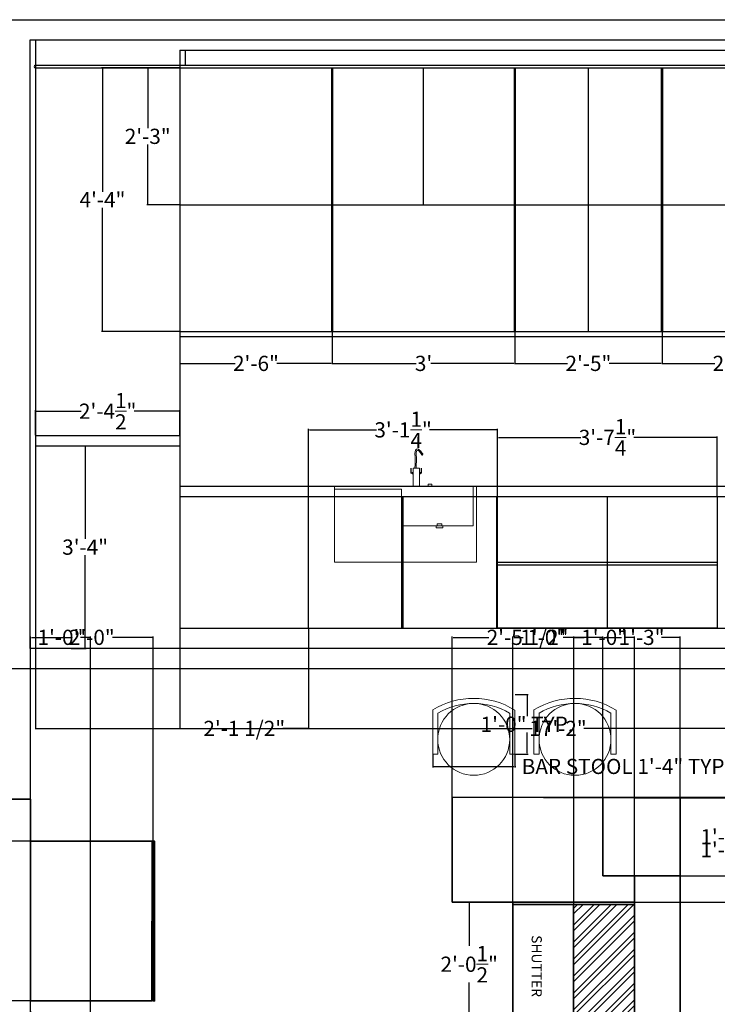
# Model space of a CAD drawing. Units: inches. Extents: x 1686244 to 1686928, y 1936095 to 1936489.
# Tile 8 of 11: x 1686478 to 1686616, y 1936281 to 1936475. Entities that reach past the tile are written whole.
import ezdxf

# ---------------------------------------------------------------- set-up
doc = ezdxf.new("R2010")
doc.units = ezdxf.units.IN
doc.header["$MEASUREMENT"] = 0
for name, color, linetype, lineweight in [('A-ANNO-DIMS', 240, 'Continuous', 18), ('A-ANNO-TEXT', 7, 'Continuous', 18), ('A-CASE', 7, 'Continuous', 35), ('A-ELEV', 7, 'Continuous', 25), ('A-FLOR-PATT', 252, 'Continuous', 13), ('A-FURN', 40, 'Continuous', 18)]:
    doc.layers.add(name, color=color, linetype=linetype, lineweight=lineweight)
doc.styles.get("Standard").update_dxf_attribs({"font": 'arial.ttf'})
doc.dimstyles.get("Standard").update_dxf_attribs({"dimtxt": 3, "dimasz": 0.18, "dimexe": 0.18, "dimexo": 0.0625, "dimgap": 0.09, "dimtad": 0, "dimtih": 1, "dimtoh": 1, "dimzin": 0, "dimdsep": 46, "dimlunit": 4, "dimtxsty": 'Standard', "dimcen": 0.09, "dimadec": 0, "dimazin": 0, "dimtfac": 1, "dimtofl": 0, "dimtmove": 0, "dimatfit": 3, "dimfxl": 1, "dimtolj": 1, "dimtzin": 0, "dimarcsym": 0})

# ---------------------------------------------------------------- blocks, each defined once
blk = doc.blocks.new('*D10')
at = {"layer": 'A-ANNO-DIMS', "color": 0, "lineweight": -2, "transparency": 16777216}
for p, q in [((1686488.94, 1936390.86), (1686491.24, 1936390.86)), ((1686491.06, 1936390.68), (1686491.06, 1936372.49)), ((1686491.06, 1936351.04), (1686491.06, 1936369.24)), ((1686488.32, 1936350.86), (1686491.24, 1936350.86))]:
    blk.add_line(p, q, dxfattribs=at)
at = {"layer": 'A-ANNO-DIMS', "color": 0, "transparency": 16777216}
for points in [[(1686491.03, 1936390.68), (1686491.09, 1936390.68), (1686491.06, 1936390.86)], [(1686491.03, 1936351.04), (1686491.09, 1936351.04), (1686491.06, 1936350.86)]]:
    blk.add_solid(points, dxfattribs=at)
at = {"layer": 'Defpoints', "color": 0, "transparency": 16777216}
for p in [(1686488.88, 1936390.86), (1686491.06, 1936390.86), (1686488.26, 1936350.86)]:
    blk.add_point(p, dxfattribs=at)
at = {"layer": 'A-ANNO-DIMS', "color": 0, "transparency": 16777216, "insert": (1686491.06, 1936370.86), "char_height": 3, "attachment_point": 5}
blk.add_mtext('\\A1;3\'-4"', dxfattribs=at)
blk = doc.blocks.new('*D11')
at = {"layer": 'A-ANNO-DIMS', "color": 0, "lineweight": -2, "transparency": 16777216}
for p, q in [((1686509.7, 1936465.36), (1686494.3, 1936465.36)), ((1686494.48, 1936465.18), (1686494.48, 1936440.95)), ((1686494.48, 1936413.54), (1686494.48, 1936437.77)), ((1686509.7, 1936413.36), (1686494.3, 1936413.36))]:
    blk.add_line(p, q, dxfattribs=at)
at = {"layer": 'A-ANNO-DIMS', "color": 0, "transparency": 16777216}
for points in [[(1686494.45, 1936465.18), (1686494.51, 1936465.18), (1686494.48, 1936465.36)], [(1686494.45, 1936413.54), (1686494.51, 1936413.54), (1686494.48, 1936413.36)]]:
    blk.add_solid(points, dxfattribs=at)
at = {"layer": 'Defpoints', "color": 0, "transparency": 16777216}
for p in [(1686509.76, 1936465.36), (1686494.48, 1936413.36), (1686509.76, 1936413.36)]:
    blk.add_point(p, dxfattribs=at)
at = {"layer": 'A-ANNO-DIMS', "color": 0, "transparency": 16777216, "insert": (1686494.48, 1936439.36), "char_height": 3, "attachment_point": 5}
blk.add_mtext('\\A1;4\'-4"', dxfattribs=at)
blk = doc.blocks.new('*D12')
at = {"layer": 'A-ANNO-DIMS', "color": 0, "lineweight": -2, "transparency": 16777216}
for p, q in [((1686509.63, 1936465.36), (1686503.22, 1936465.36)), ((1686503.4, 1936465.18), (1686503.4, 1936453.49)), ((1686503.4, 1936438.54), (1686503.4, 1936450.24)), ((1686509.7, 1936438.36), (1686503.22, 1936438.36))]:
    blk.add_line(p, q, dxfattribs=at)
at = {"layer": 'A-ANNO-DIMS', "color": 0, "transparency": 16777216}
for points in [[(1686503.37, 1936465.18), (1686503.43, 1936465.18), (1686503.4, 1936465.36)], [(1686503.37, 1936438.54), (1686503.43, 1936438.54), (1686503.4, 1936438.36)]]:
    blk.add_solid(points, dxfattribs=at)
at = {"layer": 'Defpoints', "color": 0, "transparency": 16777216}
for p in [(1686503.4, 1936465.36), (1686509.7, 1936465.36), (1686509.76, 1936438.36)]:
    blk.add_point(p, dxfattribs=at)
at = {"layer": 'A-ANNO-DIMS', "color": 0, "transparency": 16777216, "insert": (1686503.4, 1936451.86), "char_height": 3, "attachment_point": 5}
blk.add_mtext('\\A1;2\'-3"', dxfattribs=at)
blk = doc.blocks.new('*D13')
at = {"layer": 'A-ANNO-DIMS', "color": 0, "lineweight": -2, "transparency": 16777216}
for p, q in [((1686509.7, 1936413.3), (1686509.7, 1936406.91)), ((1686539.76, 1936413.3), (1686539.76, 1936406.91)), ((1686509.88, 1936407.09), (1686520.62, 1936407.09)), ((1686539.58, 1936407.09), (1686528.83, 1936407.09))]:
    blk.add_line(p, q, dxfattribs=at)
at = {"layer": 'A-ANNO-DIMS', "color": 0, "transparency": 16777216}
for points in [[(1686509.88, 1936407.12), (1686509.88, 1936407.06), (1686509.7, 1936407.09)], [(1686539.58, 1936407.12), (1686539.58, 1936407.06), (1686539.76, 1936407.09)]]:
    blk.add_solid(points, dxfattribs=at)
at = {"layer": 'Defpoints', "color": 0, "transparency": 16777216}
for p in [(1686509.7, 1936413.36), (1686539.76, 1936413.36), (1686539.76, 1936407.09)]:
    blk.add_point(p, dxfattribs=at)
at = {"layer": 'A-ANNO-DIMS', "color": 0, "transparency": 16777216, "insert": (1686524.73, 1936407.09), "char_height": 3, "attachment_point": 5}
blk.add_mtext('\\A1;2\'-6"', dxfattribs=at)
blk = doc.blocks.new('*D14')
at = {"layer": 'A-ANNO-DIMS', "color": 0, "lineweight": -2, "transparency": 16777216}
for p, q in [((1686539.76, 1936413.3), (1686539.76, 1936406.91)), ((1686575.76, 1936413.3), (1686575.76, 1936406.91)), ((1686539.94, 1936407.09), (1686556.29, 1936407.09)), ((1686575.58, 1936407.09), (1686559.23, 1936407.09))]:
    blk.add_line(p, q, dxfattribs=at)
at = {"layer": 'A-ANNO-DIMS', "color": 0, "transparency": 16777216}
for points in [[(1686539.94, 1936407.12), (1686539.94, 1936407.06), (1686539.76, 1936407.09)], [(1686575.58, 1936407.12), (1686575.58, 1936407.06), (1686575.76, 1936407.09)]]:
    blk.add_solid(points, dxfattribs=at)
at = {"layer": 'Defpoints', "color": 0, "transparency": 16777216}
for p in [(1686539.76, 1936413.36), (1686575.76, 1936413.36), (1686575.76, 1936407.09)]:
    blk.add_point(p, dxfattribs=at)
at = {"layer": 'A-ANNO-DIMS', "color": 0, "transparency": 16777216, "insert": (1686557.76, 1936407.09), "char_height": 3, "attachment_point": 5}
blk.add_mtext("\\A1;3'", dxfattribs=at)
blk = doc.blocks.new('*D15')
at = {"layer": 'A-ANNO-DIMS', "color": 0, "lineweight": -2, "transparency": 16777216}
for p, q in [((1686575.76, 1936413.3), (1686575.76, 1936406.91)), ((1686604.76, 1936413.3), (1686604.76, 1936406.91)), ((1686575.94, 1936407.09), (1686586.16, 1936407.09)), ((1686604.58, 1936407.09), (1686594.36, 1936407.09))]:
    blk.add_line(p, q, dxfattribs=at)
at = {"layer": 'A-ANNO-DIMS', "color": 0, "transparency": 16777216}
for points in [[(1686575.94, 1936407.12), (1686575.94, 1936407.06), (1686575.76, 1936407.09)], [(1686604.58, 1936407.12), (1686604.58, 1936407.06), (1686604.76, 1936407.09)]]:
    blk.add_solid(points, dxfattribs=at)
at = {"layer": 'Defpoints', "color": 0, "transparency": 16777216}
for p in [(1686575.76, 1936413.36), (1686604.76, 1936413.36), (1686604.76, 1936407.09)]:
    blk.add_point(p, dxfattribs=at)
at = {"layer": 'A-ANNO-DIMS', "color": 0, "transparency": 16777216, "insert": (1686590.26, 1936407.09), "char_height": 3, "attachment_point": 5}
blk.add_mtext('\\A1;2\'-5"', dxfattribs=at)
blk = doc.blocks.new('*D16')
at = {"layer": 'A-ANNO-DIMS', "color": 0, "lineweight": -2, "transparency": 16777216}
for p, q in [((1686604.76, 1936413.3), (1686604.76, 1936406.91)), ((1686633.76, 1936413.3), (1686633.76, 1936406.91)), ((1686604.94, 1936407.09), (1686615.16, 1936407.09)), ((1686633.58, 1936407.09), (1686623.36, 1936407.09))]:
    blk.add_line(p, q, dxfattribs=at)
at = {"layer": 'A-ANNO-DIMS', "color": 0, "transparency": 16777216}
for points in [[(1686604.94, 1936407.12), (1686604.94, 1936407.06), (1686604.76, 1936407.09)], [(1686633.58, 1936407.12), (1686633.58, 1936407.06), (1686633.76, 1936407.09)]]:
    blk.add_solid(points, dxfattribs=at)
at = {"layer": 'Defpoints', "color": 0, "transparency": 16777216}
for p in [(1686604.76, 1936413.36), (1686633.76, 1936413.36), (1686633.76, 1936407.09)]:
    blk.add_point(p, dxfattribs=at)
at = {"layer": 'A-ANNO-DIMS', "color": 0, "transparency": 16777216, "insert": (1686619.26, 1936407.09), "char_height": 3, "attachment_point": 5}
blk.add_mtext('\\A1;2\'-5"', dxfattribs=at)
blk = doc.blocks.new('*D55')
at = {"layer": 'A-ANNO-DIMS', "color": 0, "lineweight": -2, "transparency": 16777216}
for p, q in [((1686575.28, 1936300.86), (1686566.58, 1936300.86)), ((1686566.76, 1936300.68), (1686566.76, 1936292.24)), ((1686566.76, 1936276.54), (1686566.76, 1936284.99)), ((1686575.22, 1936276.36), (1686566.58, 1936276.36))]:
    blk.add_line(p, q, dxfattribs=at)
at = {"layer": 'A-ANNO-DIMS', "color": 0, "transparency": 16777216}
for points in [[(1686566.73, 1936300.68), (1686566.79, 1936300.68), (1686566.76, 1936300.86)], [(1686566.73, 1936276.54), (1686566.79, 1936276.54), (1686566.76, 1936276.36)]]:
    blk.add_solid(points, dxfattribs=at)
at = {"layer": 'Defpoints', "color": 0, "transparency": 16777216}
for p in [(1686566.76, 1936300.86), (1686575.35, 1936300.86), (1686575.28, 1936276.36)]:
    blk.add_point(p, dxfattribs=at)
at = {"layer": 'A-ANNO-DIMS', "color": 0, "transparency": 16777216, "insert": (1686566.76, 1936288.61), "char_height": 3, "attachment_point": 5}
blk.add_mtext('\\A1;2\'-0{\\H1x;\\S1/2;}"', dxfattribs=at)
blk = doc.blocks.new('*D58')
at = {"layer": 'A-ANNO-DIMS', "color": 0, "lineweight": -2, "transparency": 16777216}
for p, q in [((1686481.26, 1936392.93), (1686481.26, 1936397.84)), ((1686481.44, 1936397.66), (1686490.31, 1936397.66)), ((1686509.58, 1936397.66), (1686500.7, 1936397.66)), ((1686509.76, 1936392.93), (1686509.76, 1936397.84))]:
    blk.add_line(p, q, dxfattribs=at)
at = {"layer": 'A-ANNO-DIMS', "color": 0, "transparency": 16777216}
for points in [[(1686481.44, 1936397.69), (1686481.44, 1936397.63), (1686481.26, 1936397.66)], [(1686509.58, 1936397.69), (1686509.58, 1936397.63), (1686509.76, 1936397.66)]]:
    blk.add_solid(points, dxfattribs=at)
at = {"layer": 'Defpoints', "color": 0, "transparency": 16777216}
for p in [(1686509.76, 1936397.66), (1686481.26, 1936392.86), (1686509.76, 1936392.86)]:
    blk.add_point(p, dxfattribs=at)
at = {"layer": 'A-ANNO-DIMS', "color": 0, "transparency": 16777216, "insert": (1686495.51, 1936397.66), "char_height": 3, "attachment_point": 5}
blk.add_mtext('\\A1;2\'-4{\\H1x;\\S1/2;}"', dxfattribs=at)
blk = doc.blocks.new('*D59')
at = {"layer": 'A-ANNO-DIMS', "color": 0, "lineweight": -2, "transparency": 16777216}
for p, q in [((1686535.11, 1936380.93), (1686535.11, 1936394.16)), ((1686535.29, 1936393.98), (1686548.52, 1936393.98)), ((1686572.18, 1936393.98), (1686558.95, 1936393.98)), ((1686572.36, 1936380.93), (1686572.36, 1936394.16))]:
    blk.add_line(p, q, dxfattribs=at)
at = {"layer": 'A-ANNO-DIMS', "color": 0, "transparency": 16777216}
for points in [[(1686535.29, 1936394.01), (1686535.29, 1936393.95), (1686535.11, 1936393.98)], [(1686572.18, 1936394.01), (1686572.18, 1936393.95), (1686572.36, 1936393.98)]]:
    blk.add_solid(points, dxfattribs=at)
at = {"layer": 'Defpoints', "color": 0, "transparency": 16777216}
for p in [(1686572.36, 1936393.98), (1686535.11, 1936380.86), (1686572.36, 1936380.86)]:
    blk.add_point(p, dxfattribs=at)
at = {"layer": 'A-ANNO-DIMS', "color": 0, "transparency": 16777216, "insert": (1686553.73, 1936393.98), "char_height": 3, "attachment_point": 5}
blk.add_mtext('\\A1;3\'-1{\\H1x;\\S1/4;}"', dxfattribs=at)
blk = doc.blocks.new('*D60')
at = {"layer": 'A-ANNO-DIMS', "color": 0, "lineweight": -2, "transparency": 16777216}
for p, q in [((1686572.36, 1936380.93), (1686572.36, 1936392.68)), ((1686572.54, 1936392.5), (1686588.79, 1936392.5)), ((1686615.48, 1936392.5), (1686599.22, 1936392.5)), ((1686615.66, 1936380.93), (1686615.66, 1936392.68))]:
    blk.add_line(p, q, dxfattribs=at)
at = {"layer": 'A-ANNO-DIMS', "color": 0, "transparency": 16777216}
for points in [[(1686572.54, 1936392.53), (1686572.54, 1936392.47), (1686572.36, 1936392.5)], [(1686615.48, 1936392.53), (1686615.48, 1936392.47), (1686615.66, 1936392.5)]]:
    blk.add_solid(points, dxfattribs=at)
at = {"layer": 'Defpoints', "color": 0, "transparency": 16777216}
for p in [(1686615.66, 1936392.5), (1686572.36, 1936380.86), (1686615.66, 1936380.86)]:
    blk.add_point(p, dxfattribs=at)
at = {"layer": 'A-ANNO-DIMS', "color": 0, "transparency": 16777216, "insert": (1686594.01, 1936392.5), "char_height": 3, "attachment_point": 5}
blk.add_mtext('\\A1;3\'-7{\\H1x;\\S1/4;}"', dxfattribs=at)
blk = doc.blocks.new('BAR-STOOL')
for p, q in [((0, 8.74), (0, 0)), ((1, 0), (1, 8.08)), ((15.17, 0), (15.17, 8.08)), ((16.17, 7.08), (16.17, 8.68)), ((16.17, 0), (16.17, 7.08)), ((0, 0), (1, 0)), ((15.17, 0), (16.17, 0))]:
    blk.add_line(p, q)
for centre, radius, start, end in [((8.03, -4.44), 15.44, 58.1962, 121.3464), ((8.08, -4.09), 14.08, 59.7979, 120.2021)]:
    blk.add_arc(centre, radius, start, end)
blk = doc.blocks.new('*D67')
at = {"layer": 'A-ANNO-DIMS', "color": 0, "lineweight": -2, "transparency": 16777216}
for p, q in [((1686559.57, 1936329.98), (1686559.57, 1936327.43)), ((1686575.74, 1936329.98), (1686575.74, 1936327.43)), ((1686559.75, 1936327.61), (1686575.56, 1936327.61)), ((1686575.74, 1936327.61), (1686575.92, 1936327.61))]:
    blk.add_line(p, q, dxfattribs=at)
at = {"layer": 'A-ANNO-DIMS', "color": 0, "transparency": 16777216}
for points in [[(1686559.75, 1936327.64), (1686559.75, 1936327.58), (1686559.57, 1936327.61)], [(1686575.56, 1936327.64), (1686575.56, 1936327.58), (1686575.74, 1936327.61)]]:
    blk.add_solid(points, dxfattribs=at)
at = {"layer": 'Defpoints', "color": 0, "transparency": 16777216}
for p in [(1686559.57, 1936330.04), (1686575.74, 1936330.04), (1686575.74, 1936327.61)]:
    blk.add_point(p, dxfattribs=at)
at = {"layer": 'A-ANNO-DIMS', "color": 0, "transparency": 16777216, "insert": (1686597.66, 1936327.61), "char_height": 3, "attachment_point": 5}
blk.add_mtext('\\A1;BAR STOOL 1\'-4" TYP.', dxfattribs=at)
blk = doc.blocks.new('*D68')
at = {"layer": 'A-ANNO-DIMS', "color": 0, "lineweight": -2, "transparency": 16777216}
for p, q in [((1686575.8, 1936341.81), (1686578.35, 1936341.81)), ((1686578.17, 1936341.63), (1686578.17, 1936337.55)), ((1686578.17, 1936330.22), (1686578.17, 1936334.3)), ((1686575.8, 1936330.04), (1686578.35, 1936330.04))]:
    blk.add_line(p, q, dxfattribs=at)
at = {"layer": 'A-ANNO-DIMS', "color": 0, "transparency": 16777216}
for points in [[(1686578.14, 1936341.63), (1686578.2, 1936341.63), (1686578.17, 1936341.81)], [(1686578.14, 1936330.22), (1686578.2, 1936330.22), (1686578.17, 1936330.04)]]:
    blk.add_solid(points, dxfattribs=at)
at = {"layer": 'Defpoints', "color": 0, "transparency": 16777216}
for p in [(1686575.74, 1936341.81), (1686578.17, 1936341.81), (1686575.74, 1936330.04)]:
    blk.add_point(p, dxfattribs=at)
at = {"layer": 'A-ANNO-DIMS', "color": 0, "transparency": 16777216, "insert": (1686578.17, 1936335.93), "char_height": 3, "attachment_point": 5}
blk.add_mtext('\\A1;1\'-0" TYP.', dxfattribs=at)
blk = doc.blocks.new('*D97')
at = {"layer": 'A-ANNO-DIMS', "color": 0, "lineweight": -2, "transparency": 16777216}
for p, q in [((1686481.26, 1936350.8), (1686481.26, 1936334.93)), ((1686687.26, 1936350.8), (1686687.26, 1936334.93)), ((1686481.44, 1936335.11), (1686579.16, 1936335.11)), ((1686687.08, 1936335.11), (1686589.36, 1936335.11))]:
    blk.add_line(p, q, dxfattribs=at)
at = {"layer": 'A-ANNO-DIMS', "color": 0, "transparency": 16777216}
for points in [[(1686481.44, 1936335.14), (1686481.44, 1936335.08), (1686481.26, 1936335.11)], [(1686687.08, 1936335.14), (1686687.08, 1936335.08), (1686687.26, 1936335.11)]]:
    blk.add_solid(points, dxfattribs=at)
at = {"layer": 'Defpoints', "color": 0, "transparency": 16777216}
for p in [(1686481.26, 1936350.86), (1686687.26, 1936350.86), (1686687.26, 1936335.11)]:
    blk.add_point(p, dxfattribs=at)
at = {"layer": 'A-ANNO-DIMS', "color": 0, "transparency": 16777216, "insert": (1686584.26, 1936335.11), "char_height": 3, "attachment_point": 5}
blk.add_mtext('\\A1;17\'-2"', dxfattribs=at)
blk = doc.blocks.new('*D98')
at = {"layer": 'A-ANNO-DIMS', "color": 0, "lineweight": -2, "transparency": 16777216}
for p, q in [((1686509.76, 1936354.8), (1686509.76, 1936334.93)), ((1686535.11, 1936354.8), (1686535.11, 1936334.93)), ((1686509.94, 1936335.11), (1686514.84, 1936335.11)), ((1686534.93, 1936335.11), (1686530.03, 1936335.11))]:
    blk.add_line(p, q, dxfattribs=at)
at = {"layer": 'A-ANNO-DIMS', "color": 0, "transparency": 16777216}
for points in [[(1686509.94, 1936335.14), (1686509.94, 1936335.08), (1686509.76, 1936335.11)], [(1686534.93, 1936335.14), (1686534.93, 1936335.08), (1686535.11, 1936335.11)]]:
    blk.add_solid(points, dxfattribs=at)
at = {"layer": 'Defpoints', "color": 0, "transparency": 16777216}
for p in [(1686509.76, 1936354.86), (1686535.11, 1936354.86), (1686535.11, 1936335.11)]:
    blk.add_point(p, dxfattribs=at)
at = {"layer": 'A-ANNO-DIMS', "color": 0, "transparency": 16777216, "insert": (1686522.43, 1936335.11), "char_height": 3, "attachment_point": 5}
blk.add_mtext('\\A1;2\'-1 1/2"', dxfattribs=at)
blk = doc.blocks.new('*D116')
at = {"layer": 'A-ANNO-DIMS', "color": 0, "lineweight": -2, "transparency": 16777216}
for p, q in [((1686480.29, 1936207.43), (1686480.29, 1936353.25)), ((1686480.47, 1936353.07), (1686482.26, 1936353.07)), ((1686491.93, 1936353.07), (1686490.14, 1936353.07)), ((1686492.11, 1936207.43), (1686492.11, 1936353.25))]:
    blk.add_line(p, q, dxfattribs=at)
at = {"layer": 'A-ANNO-DIMS', "color": 0, "transparency": 16777216}
for points in [[(1686480.47, 1936353.1), (1686480.47, 1936353.04), (1686480.29, 1936353.07)], [(1686491.93, 1936353.1), (1686491.93, 1936353.04), (1686492.11, 1936353.07)]]:
    blk.add_solid(points, dxfattribs=at)
at = {"layer": 'Defpoints', "color": 0, "transparency": 16777216}
for p in [(1686492.11, 1936353.07), (1686480.29, 1936207.36), (1686492.11, 1936207.36)]:
    blk.add_point(p, dxfattribs=at)
at = {"layer": 'A-ANNO-DIMS', "color": 0, "transparency": 16777216, "insert": (1686486.2, 1936353.07), "char_height": 3, "attachment_point": 5}
blk.add_mtext('\\A1;1\'-0"', dxfattribs=at)
blk = doc.blocks.new('*D117')
at = {"layer": 'A-ANNO-DIMS', "color": 0, "lineweight": -2, "transparency": 16777216}
for p, q in [((1686575.35, 1936300.93), (1686575.35, 1936353.25)), ((1686575.53, 1936353.07), (1686577.41, 1936353.07)), ((1686587.17, 1936353.07), (1686585.28, 1936353.07)), ((1686587.35, 1936300.43), (1686587.35, 1936353.25))]:
    blk.add_line(p, q, dxfattribs=at)
at = {"layer": 'A-ANNO-DIMS', "color": 0, "transparency": 16777216}
for points in [[(1686575.53, 1936353.1), (1686575.53, 1936353.04), (1686575.35, 1936353.07)], [(1686587.17, 1936353.1), (1686587.17, 1936353.04), (1686587.35, 1936353.07)]]:
    blk.add_solid(points, dxfattribs=at)
at = {"layer": 'Defpoints', "color": 0, "transparency": 16777216}
for p in [(1686587.35, 1936353.07), (1686575.35, 1936300.86), (1686587.35, 1936300.36)]:
    blk.add_point(p, dxfattribs=at)
at = {"layer": 'A-ANNO-DIMS', "color": 0, "transparency": 16777216, "insert": (1686581.35, 1936353.07), "char_height": 3, "attachment_point": 5}
blk.add_mtext('\\A1;1\'-0"', dxfattribs=at)
blk = doc.blocks.new('*D118')
at = {"layer": 'A-ANNO-DIMS', "color": 0, "lineweight": -2, "transparency": 16777216}
for p, q in [((1686587.35, 1936300.43), (1686587.35, 1936353.25)), ((1686587.53, 1936353.07), (1686589.41, 1936353.07)), ((1686599.17, 1936353.07), (1686597.28, 1936353.07)), ((1686599.35, 1936300.93), (1686599.35, 1936353.25))]:
    blk.add_line(p, q, dxfattribs=at)
at = {"layer": 'A-ANNO-DIMS', "color": 0, "transparency": 16777216}
for points in [[(1686587.53, 1936353.1), (1686587.53, 1936353.04), (1686587.35, 1936353.07)], [(1686599.17, 1936353.1), (1686599.17, 1936353.04), (1686599.35, 1936353.07)]]:
    blk.add_solid(points, dxfattribs=at)
at = {"layer": 'Defpoints', "color": 0, "transparency": 16777216}
for p in [(1686599.35, 1936353.07), (1686587.35, 1936300.36), (1686599.35, 1936300.86)]:
    blk.add_point(p, dxfattribs=at)
at = {"layer": 'A-ANNO-DIMS', "color": 0, "transparency": 16777216, "insert": (1686593.35, 1936353.07), "char_height": 3, "attachment_point": 5}
blk.add_mtext('\\A1;1\'-0"', dxfattribs=at)
blk = doc.blocks.new('*D120')
at = {"layer": 'A-ANNO-DIMS', "color": 0, "lineweight": -2, "transparency": 16777216}
for p, q in [((1686599.41, 1936300.86), (1686620.56, 1936300.86)), ((1686620.38, 1936300.68), (1686620.38, 1936215.99)), ((1686620.38, 1936128.04), (1686620.38, 1936212.74)), ((1686599.41, 1936127.86), (1686620.56, 1936127.86))]:
    blk.add_line(p, q, dxfattribs=at)
at = {"layer": 'A-ANNO-DIMS', "color": 0, "transparency": 16777216}
for points in [[(1686620.35, 1936300.68), (1686620.41, 1936300.68), (1686620.38, 1936300.86)], [(1686620.35, 1936128.04), (1686620.41, 1936128.04), (1686620.38, 1936127.86)]]:
    blk.add_solid(points, dxfattribs=at)
at = {"layer": 'Defpoints', "color": 0, "transparency": 16777216}
for p in [(1686599.35, 1936300.86), (1686599.35, 1936127.86), (1686620.38, 1936127.86)]:
    blk.add_point(p, dxfattribs=at)
at = {"layer": 'A-ANNO-DIMS', "color": 0, "transparency": 16777216, "insert": (1686620.38, 1936214.36), "char_height": 3, "attachment_point": 5}
blk.add_mtext('\\A1;14\'-5"', dxfattribs=at)
blk = doc.blocks.new('*D121')
at = {"layer": 'A-ANNO-DIMS', "color": 0, "lineweight": -2, "transparency": 16777216}
for p, q in [((1686480.29, 1936312.93), (1686480.29, 1936353.25)), ((1686480.47, 1936353.07), (1686488.27, 1936353.07)), ((1686504.28, 1936353.07), (1686496.48, 1936353.07)), ((1686504.46, 1936312.93), (1686504.46, 1936353.25))]:
    blk.add_line(p, q, dxfattribs=at)
at = {"layer": 'A-ANNO-DIMS', "color": 0, "transparency": 16777216}
for points in [[(1686480.47, 1936353.1), (1686480.47, 1936353.04), (1686480.29, 1936353.07)], [(1686504.28, 1936353.1), (1686504.28, 1936353.04), (1686504.46, 1936353.07)]]:
    blk.add_solid(points, dxfattribs=at)
at = {"layer": 'Defpoints', "color": 0, "transparency": 16777216}
for p in [(1686504.46, 1936353.07), (1686480.29, 1936312.86), (1686504.46, 1936312.86)]:
    blk.add_point(p, dxfattribs=at)
at = {"layer": 'A-ANNO-DIMS', "color": 0, "transparency": 16777216, "insert": (1686492.37, 1936353.07), "char_height": 3, "attachment_point": 5}
blk.add_mtext('\\A1;2\'-0"', dxfattribs=at)
blk = doc.blocks.new('*D122')
at = {"layer": 'A-ANNO-DIMS', "color": 0, "lineweight": -2, "transparency": 16777216}
for p, q in [((1686504.4, 1936312.86), (1686459.08, 1936312.86)), ((1686459.26, 1936312.68), (1686459.26, 1936298.75)), ((1686459.26, 1936281.54), (1686459.26, 1936295.47)), ((1686504.4, 1936281.36), (1686459.08, 1936281.36))]:
    blk.add_line(p, q, dxfattribs=at)
at = {"layer": 'A-ANNO-DIMS', "color": 0, "transparency": 16777216}
for points in [[(1686459.23, 1936312.68), (1686459.29, 1936312.68), (1686459.26, 1936312.86)], [(1686459.23, 1936281.54), (1686459.29, 1936281.54), (1686459.26, 1936281.36)]]:
    blk.add_solid(points, dxfattribs=at)
at = {"layer": 'Defpoints', "color": 0, "transparency": 16777216}
for p in [(1686504.46, 1936312.86), (1686459.26, 1936281.36), (1686504.46, 1936281.36)]:
    blk.add_point(p, dxfattribs=at)
at = {"layer": 'A-ANNO-DIMS', "color": 0, "transparency": 16777216, "insert": (1686459.26, 1936297.11), "char_height": 3, "attachment_point": 5}
blk.add_mtext('\\A1;2\'-7 1/2"', dxfattribs=at)
blk = doc.blocks.new('*D123')
at = {"layer": 'A-ANNO-DIMS', "color": 0, "lineweight": -2, "transparency": 16777216}
for p, q in [((1686563.41, 1936321.6), (1686563.41, 1936353.25)), ((1686563.59, 1936353.07), (1686570.66, 1936353.07)), ((1686592.93, 1936353.07), (1686585.86, 1936353.07)), ((1686593.11, 1936321.53), (1686593.11, 1936353.25))]:
    blk.add_line(p, q, dxfattribs=at)
at = {"layer": 'A-ANNO-DIMS', "color": 0, "transparency": 16777216}
for points in [[(1686563.59, 1936353.1), (1686563.59, 1936353.04), (1686563.41, 1936353.07)], [(1686592.93, 1936353.1), (1686592.93, 1936353.04), (1686593.11, 1936353.07)]]:
    blk.add_solid(points, dxfattribs=at)
at = {"layer": 'Defpoints', "color": 0, "transparency": 16777216}
for p in [(1686593.11, 1936353.07), (1686563.41, 1936321.54), (1686593.11, 1936321.46)]:
    blk.add_point(p, dxfattribs=at)
at = {"layer": 'A-ANNO-DIMS', "color": 0, "transparency": 16777216, "insert": (1686578.26, 1936353.07), "char_height": 3, "attachment_point": 5}
blk.add_mtext('\\A1;2\'-5 1/2"', dxfattribs=at)
blk = doc.blocks.new('*D124')
at = {"layer": 'A-ANNO-DIMS', "color": 0, "lineweight": -2, "transparency": 16777216}
for p, q in [((1686593.11, 1936321.53), (1686593.11, 1936353.25)), ((1686593.29, 1936353.07), (1686596.79, 1936353.07)), ((1686608.17, 1936353.07), (1686604.66, 1936353.07)), ((1686608.35, 1936321.51), (1686608.35, 1936353.25))]:
    blk.add_line(p, q, dxfattribs=at)
at = {"layer": 'A-ANNO-DIMS', "color": 0, "transparency": 16777216}
for points in [[(1686593.29, 1936353.1), (1686593.29, 1936353.04), (1686593.11, 1936353.07)], [(1686608.17, 1936353.1), (1686608.17, 1936353.04), (1686608.35, 1936353.07)]]:
    blk.add_solid(points, dxfattribs=at)
at = {"layer": 'Defpoints', "color": 0, "transparency": 16777216}
for p in [(1686608.35, 1936353.07), (1686593.11, 1936321.46), (1686608.35, 1936321.45)]:
    blk.add_point(p, dxfattribs=at)
at = {"layer": 'A-ANNO-DIMS', "color": 0, "transparency": 16777216, "insert": (1686600.73, 1936353.07), "char_height": 3, "attachment_point": 5}
blk.add_mtext('\\A1;1\'-3"', dxfattribs=at)
blk = doc.blocks.new('*D125')
at = {"layer": 'A-ANNO-DIMS', "color": 0, "lineweight": -2, "transparency": 16777216}
for p, q in [((1686563.48, 1936321.54), (1686620.56, 1936321.54)), ((1686620.38, 1936321.36), (1686620.38, 1936312.84)), ((1686620.38, 1936301.04), (1686620.38, 1936309.56)), ((1686563.48, 1936300.86), (1686620.56, 1936300.86))]:
    blk.add_line(p, q, dxfattribs=at)
at = {"layer": 'A-ANNO-DIMS', "color": 0, "transparency": 16777216}
for points in [[(1686620.35, 1936321.36), (1686620.41, 1936321.36), (1686620.38, 1936321.54)], [(1686620.35, 1936301.04), (1686620.41, 1936301.04), (1686620.38, 1936300.86)]]:
    blk.add_solid(points, dxfattribs=at)
at = {"layer": 'Defpoints', "color": 0, "transparency": 16777216}
for p in [(1686563.41, 1936321.54), (1686563.41, 1936300.86), (1686620.38, 1936300.86)]:
    blk.add_point(p, dxfattribs=at)
at = {"layer": 'A-ANNO-DIMS', "color": 0, "transparency": 16777216, "insert": (1686620.38, 1936311.2), "char_height": 3, "attachment_point": 5}
blk.add_mtext('\\A1;1\'-8 1/2"', dxfattribs=at)
blk = doc.blocks.new('*D126')
at = {"layer": 'A-ANNO-DIMS', "color": 0, "lineweight": -2, "transparency": 16777216}
for p, q in [((1686608.41, 1936321.45), (1686620.56, 1936321.45)), ((1686620.38, 1936321.27), (1686620.38, 1936315.38)), ((1686620.38, 1936306.21), (1686620.38, 1936312.1)), ((1686608.39, 1936306.03), (1686620.56, 1936306.03))]:
    blk.add_line(p, q, dxfattribs=at)
at = {"layer": 'A-ANNO-DIMS', "color": 0, "transparency": 16777216}
for points in [[(1686620.35, 1936321.27), (1686620.41, 1936321.27), (1686620.38, 1936321.45)], [(1686620.35, 1936306.21), (1686620.41, 1936306.21), (1686620.38, 1936306.03)]]:
    blk.add_solid(points, dxfattribs=at)
at = {"layer": 'Defpoints', "color": 0, "transparency": 16777216}
for p in [(1686608.35, 1936321.45), (1686608.32, 1936306.03), (1686620.38, 1936306.03)]:
    blk.add_point(p, dxfattribs=at)
at = {"layer": 'A-ANNO-DIMS', "color": 0, "transparency": 16777216, "insert": (1686620.38, 1936313.74), "char_height": 3, "attachment_point": 5}
blk.add_mtext('\\A1;1\'-3 1/2"', dxfattribs=at)

msp = doc.modelspace()

# ---------------------------------------------------------------- hatches: boundary and pattern name
at = {"layer": 'A-FLOR-PATT'}
h = msp.add_hatch(dxfattribs=at)
h.set_pattern_fill('ANSI32', color=256, scale=6.3)
h.paths.add_polyline_path([(1686599.345, 1936233.864), (1686587.345, 1936233.864), (1686587.345, 1936213.864), (1686599.345, 1936213.864)])
h.paths.add_polyline_path([(1686596.539, 1936252.932, 0.4142136), (1686595.539, 1936253.932), (1686587.345, 1936253.932), (1686587.345, 1936238.182), (1686595.539, 1936238.182, 0.4142136), (1686596.539, 1936239.182)])
h.paths.add_polyline_path([(1686590.539, 1936246.182, -1), (1686588.539, 1936246.182, -1)], flags=16)
h.paths.add_polyline_path([(1686590.039, 1936246.182, -1), (1686589.039, 1936246.182, -1)], flags=0)
h.paths.add_polyline_path([(1686599.345, 1936300.364), (1686587.345, 1936300.364), (1686587.345, 1936276.864), (1686599.345, 1936276.864)])
h.paths.add_polyline_path([(1686596.539, 1936270.182, 0.4142136), (1686595.539, 1936271.182), (1686587.345, 1936271.182), (1686587.345, 1936255.432), (1686595.539, 1936255.432, 0.4142136), (1686596.539, 1936256.432)])
h.paths.add_polyline_path([(1686590.539, 1936263.182, -1), (1686588.539, 1936263.182, -1)], flags=16)
h.paths.add_polyline_path([(1686589.039, 1936263.182, -1), (1686590.039, 1936263.182, -1)], flags=0)

# ---------------------------------------------------------------- linework, layer by layer
at = {"layer": 'A-CASE'}
for p, q in [((1686471.291, 1936321.159), (1686480.291, 1936321.159)), ((1686480.291, 1936321.159), (1686480.291, 1936312.864)), ((1686593.072, 1936306.026), (1686593.109, 1936321.464)), ((1686608.345, 1936321.449), (1686599.345, 1936321.449)), ((1686608.345, 1936303.497), (1686608.345, 1936321.449)), ((1686504.458, 1936307.691), (1686504.757, 1936307.691)), ((1686504.458, 1936307.537), (1686504.757, 1936307.537)), ((1686593.072, 1936306.026), (1686608.324, 1936306.026)), ((1686599.345, 1936300.864), (1686599.345, 1936306.026)), ((1686575.345, 1936300.364), (1686599.345, 1936300.364)), ((1686587.345, 1936139.864), (1686587.345, 1936300.364)), ((1686504.227, 1936281.362), (1686480.291, 1936281.362))]:
    msp.add_line(p, q, dxfattribs=at)
for points in [[(1686608.345, 1936303.497), (1686608.345, 1936118.864), (1686471.291, 1936118.864), (1686471.291, 1936321.159)], [(1686599.345, 1936300.864), (1686563.414, 1936300.864), (1686563.414, 1936321.536), (1686599.345, 1936321.449)], [(1686480.291, 1936281.362), (1686480.291, 1936312.864), (1686504.291, 1936312.864), (1686504.205, 1936281.362)], [(1686503.85, 1936151.863), (1686524.345, 1936151.864), (1686554.345, 1936151.864), (1686564.345, 1936151.864), (1686575.345, 1936151.864), (1686575.345, 1936170.364), (1686575.345, 1936190.864), (1686575.345, 1936213.364), (1686575.345, 1936234.364), (1686575.345, 1936276.364), (1686575.345, 1936300.864), (1686599.345, 1936300.864), (1686599.345, 1936151.864), (1686599.345, 1936127.864), (1686504.291, 1936127.864), (1686480.291, 1936127.864), (1686480.291, 1936279.362)]]:
    msp.add_lwpolyline(points, dxfattribs=at)
msp.add_lwpolyline([(1686504.458, 1936312.864), (1686504.757, 1936312.864), (1686504.757, 1936281.362), (1686504.458, 1936281.362)], close=True, dxfattribs=at)
at = {"layer": 'A-ELEV'}
for p, q in [((1686481.258, 1936470.864), (1686481.258, 1936350.864)), ((1686509.758, 1936468.864), (1686509.758, 1936465.364)), ((1686509.758, 1936468.864), (1686678.258, 1936468.864)), ((1686510.758, 1936468.864), (1686510.758, 1936465.864)), ((1686481.258, 1936465.864), (1686687.259, 1936465.864)), ((1686481.258, 1936465.364), (1686687.259, 1936465.364)), ((1686509.758, 1936465.864), (1686509.758, 1936350.864)), ((1686509.758, 1936465.364), (1686509.758, 1936413.364)), ((1686557.758, 1936438.364), (1686557.758, 1936465.364)), ((1686590.258, 1936413.364), (1686590.258, 1936465.364)), ((1686509.758, 1936438.364), (1686687.259, 1936438.364)), ((1686509.758, 1936413.364), (1686687.259, 1936413.364)), ((1686509.758, 1936412.364), (1686687.259, 1936412.364)), ((1686481.258, 1936392.864), (1686509.758, 1936392.864)), ((1686481.258, 1936390.864), (1686509.758, 1936390.864)), ((1686509.758, 1936382.864), (1686687.259, 1936382.864)), ((1686509.758, 1936380.864), (1686572.358, 1936380.864)), ((1686535.108, 1936354.864), (1686535.108, 1936380.864)), ((1686553.483, 1936354.864), (1686553.483, 1936380.864)), ((1686553.733, 1936354.864), (1686553.733, 1936380.864)), ((1686572.108, 1936380.864), (1686572.108, 1936354.864)), ((1686594.008, 1936354.864), (1686594.008, 1936380.864)), ((1686615.658, 1936380.864), (1686687.259, 1936380.864)), ((1686572.358, 1936367.864), (1686615.658, 1936367.864)), ((1686572.358, 1936367.364), (1686615.658, 1936367.364)), ((1686509.758, 1936354.864), (1686687.259, 1936354.864))]:
    msp.add_line(p, q, dxfattribs=at)
for points in [[(1686691.259, 1936346.864), (1686476.258, 1936346.864), (1686476.258, 1936474.864), (1686691.259, 1936474.864)], [(1686572.358, 1936380.864), (1686615.658, 1936380.864), (1686615.658, 1936354.864), (1686572.358, 1936354.864)]]:
    msp.add_lwpolyline(points, close=True, dxfattribs=at)
msp.add_lwpolyline([(1686687.259, 1936354.864), (1686687.259, 1936350.864), (1686480.258, 1936350.864), (1686480.258, 1936470.864), (1686687.259, 1936470.864), (1686687.259, 1936412.364)], dxfattribs=at)
at = {"layer": 'A-ELEV', "const_width": 0.5}
for points in [[(1686539.758, 1936413.364), (1686539.758, 1936465.364)], [(1686575.758, 1936413.364), (1686575.758, 1936465.364)], [(1686604.758, 1936413.364), (1686604.758, 1936465.364)]]:
    msp.add_lwpolyline(points, dxfattribs=at)
at = {"layer": 'A-ELEV'}
msp.add_arc((1686481.258, 1936465.614), 0.25, 90, 270, dxfattribs=at)
at = {"layer": 'A-FURN'}
for p, q in [((1686557.406, 1936389.047), (1686557.373, 1936389.097)), ((1686555.272, 1936385.439), (1686555.272, 1936386.413)), ((1686555.45, 1936385.439), (1686555.272, 1936385.439)), ((1686555.322, 1936385.448), (1686555.322, 1936386.413)), ((1686555.45, 1936385.448), (1686555.322, 1936385.448)), ((1686557.188, 1936385.448), (1686557.316, 1936385.448)), ((1686557.188, 1936385.438), (1686557.366, 1936385.438)), ((1686557.316, 1936385.448), (1686557.316, 1936386.412)), ((1686557.366, 1936385.438), (1686557.366, 1936386.412)), ((1686567.51, 1936375.027), (1686567.51, 1936382.864)), ((1686540.205, 1936382.259), (1686553.441, 1936382.259)), ((1686553.441, 1936382.259), (1686553.441, 1936375.027)), ((1686553.441, 1936375.027), (1686567.51, 1936375.027))]:
    msp.add_line(p, q, dxfattribs=at)
for points in [[(1686555.501, 1936385.492), (1686555.45, 1936385.492), (1686555.45, 1936385.385), (1686555.501, 1936385.385)], [(1686555.685, 1936385.55), (1686555.501, 1936385.55), (1686555.501, 1936385.337), (1686555.685, 1936385.336)], [(1686555.684, 1936382.864), (1686556.954, 1936382.864), (1686556.954, 1936386.412), (1686555.684, 1936386.412)], [(1686556.954, 1936385.55), (1686557.137, 1936385.55), (1686557.137, 1936385.336), (1686556.954, 1936385.336)], [(1686557.137, 1936385.492), (1686557.188, 1936385.492), (1686557.188, 1936385.385), (1686557.137, 1936385.385)], [(1686540.205, 1936382.864), (1686568.215, 1936382.864), (1686568.215, 1936367.918), (1686540.205, 1936367.918)], [(1686558.649, 1936382.864), (1686559.371, 1936382.864), (1686559.371, 1936383.244), (1686558.649, 1936383.244)], [(1686560.224, 1936375.027), (1686561.546, 1936375.027), (1686561.546, 1936374.651), (1686560.224, 1936374.651)], [(1686560.476, 1936375.027), (1686561.355, 1936375.027), (1686561.355, 1936375.422), (1686560.476, 1936375.422)]]:
    msp.add_lwpolyline(points, close=True, dxfattribs=at)
for centre in [(1686567.656, 1936332.951), (1686587.614, 1936332.951)]:
    msp.add_circle(centre, 7.084, dxfattribs=at)
msp.add_ellipse((1686557.506, 1936389.123), major_axis=(-0.073, 0.105), ratio=0.9765064, dxfattribs=at)
for points, knots in [([(1686556.069, 1936386.419), (1686556.078, 1936386.748), (1686556.087, 1936387.076), (1686556.098, 1936387.658), (1686556.1, 1936387.913), (1686556.097, 1936388.331), (1686556.094, 1936388.495), (1686556.085, 1936388.783), (1686556.08, 1936388.907), (1686556.069, 1936389.109), (1686556.063, 1936389.187), (1686556.058, 1936389.368), (1686556.061, 1936389.47), (1686556.095, 1936389.685), (1686556.122, 1936389.793), (1686556.19, 1936389.953), (1686556.219, 1936390.01), (1686556.312, 1936390.121), (1686556.379, 1936390.172), (1686556.534, 1936390.223), (1686556.617, 1936390.22), (1686556.751, 1936390.185), (1686556.806, 1936390.155), (1686556.906, 1936390.088), (1686556.951, 1936390.049), (1686557.098, 1936389.908), (1686557.194, 1936389.786), (1686557.392, 1936389.517), (1686557.491, 1936389.37), (1686557.598, 1936389.211), (1686557.606, 1936389.199), (1686557.614, 1936389.187)], [0, 0, 0, 0, 0.97016, 0.97016, 1.738831, 1.738831, 2.2415179, 2.2415179, 2.6291018, 2.6291018, 2.8760298, 2.8760298, 3.1229577, 3.1229577, 3.3698857, 3.3698857, 3.5141943, 3.5141943, 3.6585029, 3.6585029, 3.8028115, 3.8028115, 3.9471201, 3.9471201, 4.0914287, 4.0914287, 4.4310021, 4.4310021, 4.7705755, 4.7705755, 4.7989475, 4.7989475, 4.7989475, 4.7989475]), ([(1686556.319, 1936386.412), (1686556.345, 1936387.329), (1686556.374, 1936388.371), (1686556.293, 1936389.498), (1686556.54, 1936390.34), (1686557.037, 1936389.598), (1686557.406, 1936389.047)], [0, 0, 0, 0, 2.7074617, 3.0753927, 3.5199051, 4.7989475, 4.7989475, 4.7989475, 4.7989475])]:
    msp.add_open_spline(points, degree=3, knots=knots, dxfattribs=at)

# ---------------------------------------------------------------- block references
for p in [(1686559.572, 1936330.04), (1686579.53, 1936330.04)]:
    msp.add_blockref('BAR-STOOL', p, dxfattribs=at)

# ---------------------------------------------------------------- texts
at = {"layer": 'A-ANNO-TEXT'}
msp.add_text('SHUTTER', height=2, rotation=269.96854, dxfattribs=at).set_placement((1686579.07, 1936294.335))

# ---------------------------------------------------------------- dimensions: what is measured, and where the dimension line sits
at = {"layer": 'A-ANNO-DIMS'}
for base, p1, p2, picture, middle in [((1686494.482, 1936413.364), (1686509.758, 1936465.364), (1686509.758, 1936413.364), '*D11', (1686494.482, 1936439.364)), ((1686503.402, 1936465.364), (1686509.758, 1936438.364), (1686509.696, 1936465.364), '*D12', (1686503.402, 1936451.864))]:
    dim = msp.add_linear_dim(base=base, p1=p1, p2=p2, angle=90, dimstyle='Standard', override={"dimclrd": 0, "dimclre": 0, "dimclrt": 0}, dxfattribs=at)
    dim.commit()
    dim.dimension.update_dxf_attribs({"geometry": picture, "text_midpoint": middle, "dimtype": 160})
for base, p1, p2, override, picture, middle in [((1686539.758, 1936407.086), (1686509.696, 1936413.364), (1686539.758, 1936413.364), {"dimclrd": 0, "dimclre": 0, "dimclrt": 0}, '*D13', (1686524.727, 1936407.086)), ((1686575.758, 1936407.086), (1686539.758, 1936413.364), (1686575.758, 1936413.364), {"dimclrd": 0, "dimclre": 0, "dimclrt": 0}, '*D14', (1686557.758, 1936407.086)), ((1686604.758, 1936407.086), (1686575.758, 1936413.364), (1686604.758, 1936413.364), {"dimclrd": 0, "dimclre": 0, "dimclrt": 0}, '*D15', (1686590.258, 1936407.086)), ((1686633.758, 1936407.086), (1686604.758, 1936413.364), (1686633.758, 1936413.364), {"dimclrd": 0, "dimclre": 0, "dimclrt": 0}, '*D16', (1686619.258, 1936407.086)), ((1686509.758, 1936397.664), (1686481.258, 1936392.864), (1686509.758, 1936392.864), {"dimclrd": 0, "dimclre": 0, "dimclrt": 0}, '*D58', (1686495.508, 1936397.664)), ((1686572.358, 1936393.981), (1686535.108, 1936380.864), (1686572.358, 1936380.864), {"dimclrd": 0, "dimclre": 0, "dimclrt": 0}, '*D59', (1686553.733, 1936393.981)), ((1686615.658, 1936392.502), (1686572.358, 1936380.864), (1686615.658, 1936380.864), {"dimclrd": 0, "dimclre": 0, "dimclrt": 0}, '*D60', (1686594.008, 1936392.502)), ((1686593.109, 1936353.067), (1686563.414, 1936321.536), (1686593.109, 1936321.464), {"dimdec": 1, "dimlfac": 1, "dimrnd": 0, "dimzin": 1, "dimdsep": 46, "dimlunit": 4, "dimfrac": 2}, '*D123', (1686578.262, 1936353.067)), ((1686492.108, 1936353.067), (1686480.291, 1936207.363), (1686492.108, 1936207.363), {"dimdec": 1, "dimlfac": 1, "dimrnd": 0, "dimzin": 1, "dimdsep": 46, "dimlunit": 4, "dimfrac": 2}, '*D116', (1686486.2, 1936353.067)), ((1686504.458, 1936353.067), (1686480.291, 1936312.864), (1686504.458, 1936312.864), {"dimdec": 1, "dimlfac": 1, "dimrnd": 0, "dimzin": 1, "dimdsep": 46, "dimlunit": 4, "dimfrac": 2}, '*D121', (1686492.375, 1936353.067)), ((1686535.108187, 1936335.113737), (1686509.758187, 1936354.863737), (1686535.108187, 1936354.863737), {"dimdec": 1, "dimlfac": 1, "dimrnd": 0, "dimzin": 1, "dimdsep": 46, "dimlunit": 4, "dimfrac": 2}, '*D98', (1686522.433187, 1936335.113737)), ((1686587.345, 1936353.067), (1686575.345, 1936300.864), (1686587.345, 1936300.364), {"dimdec": 1, "dimlfac": 1, "dimrnd": 0, "dimzin": 1, "dimdsep": 46, "dimlunit": 4, "dimfrac": 2}, '*D117', (1686581.345, 1936353.067)), ((1686599.345, 1936353.067), (1686587.345, 1936300.364), (1686599.345, 1936300.864), {"dimdec": 1, "dimlfac": 1, "dimrnd": 0, "dimzin": 1, "dimdsep": 46, "dimlunit": 4, "dimfrac": 2}, '*D118', (1686593.345, 1936353.067)), ((1686608.345, 1936353.067), (1686593.109, 1936321.464), (1686608.345, 1936321.449), {"dimdec": 1, "dimlfac": 1, "dimrnd": 0, "dimzin": 1, "dimdsep": 46, "dimlunit": 4, "dimfrac": 2}, '*D124', (1686600.727, 1936353.067)), ((1686687.259, 1936335.114), (1686481.258, 1936350.864), (1686687.259, 1936350.864), {"dimdec": 1, "dimlfac": 1, "dimrnd": 0, "dimzin": 1, "dimdsep": 46, "dimlunit": 4, "dimfrac": 2}, '*D97', (1686584.259, 1936335.114))]:
    dim = msp.add_linear_dim(base=base, p1=p1, p2=p2, dimstyle='Standard', override=override, dxfattribs=at)
    dim.commit()
    dim.dimension.update_dxf_attribs({"geometry": picture, "text_midpoint": middle})
for base, p1, p2, override, picture, middle in [((1686491.065, 1936390.864), (1686488.262, 1936350.864), (1686488.875, 1936390.864), {"dimclrd": 0, "dimclre": 0, "dimclrt": 0}, '*D10', (1686491.065, 1936370.864)), ((1686620.375, 1936300.864), (1686563.414, 1936321.536), (1686563.414, 1936300.864), {"dimdec": 1, "dimlfac": 1, "dimrnd": 0, "dimzin": 1, "dimdsep": 46, "dimlunit": 4, "dimfrac": 2}, '*D125', (1686620.375, 1936311.2)), ((1686620.375, 1936306.026), (1686608.345, 1936321.449), (1686608.324, 1936306.026), {"dimdec": 1, "dimlfac": 1, "dimrnd": 0, "dimzin": 1, "dimdsep": 46, "dimlunit": 4, "dimfrac": 2}, '*D126', (1686620.375, 1936313.738)), ((1686459.261, 1936281.362), (1686504.458, 1936312.864), (1686504.458, 1936281.362), {"dimdec": 1, "dimlfac": 1, "dimrnd": 0, "dimzin": 1, "dimdsep": 46, "dimlunit": 4, "dimfrac": 2}, '*D122', (1686459.261, 1936297.113)), ((1686566.76, 1936300.864), (1686575.283, 1936276.364), (1686575.345, 1936300.864), {"dimclrd": 0, "dimclre": 0, "dimclrt": 0}, '*D55', (1686566.76, 1936288.614)), ((1686620.375, 1936127.864), (1686599.345, 1936300.864), (1686599.345, 1936127.864), {"dimdec": 1, "dimlfac": 1, "dimrnd": 0, "dimzin": 1, "dimdsep": 46, "dimlunit": 4, "dimfrac": 2}, '*D120', (1686620.375, 1936214.364))]:
    dim = msp.add_linear_dim(base=base, p1=p1, p2=p2, angle=90, dimstyle='Standard', override=override, dxfattribs=at)
    dim.commit()
    dim.dimension.update_dxf_attribs({"geometry": picture, "text_midpoint": middle})
dim = msp.add_linear_dim(base=(1686578.165, 1936341.811), p1=(1686575.74, 1936330.04), p2=(1686575.74, 1936341.811), angle=90, text='<> TYP.', dimstyle='Standard', override={"dimdec": 1, "dimrnd": 0, "dimzin": 1, "dimlunit": 4, "dimfrac": 2}, dxfattribs=at)
dim.commit()
dim.dimension.update_dxf_attribs({"geometry": '*D68', "text_midpoint": (1686578.165, 1936335.925)})
dim = msp.add_linear_dim(base=(1686575.74, 1936327.614), p1=(1686559.572, 1936330.04), p2=(1686575.74, 1936330.04), text='BAR STOOL <> TYP.', dimstyle='Standard', override={"dimdec": 1, "dimrnd": 0, "dimzin": 1, "dimlunit": 4, "dimfrac": 2}, dxfattribs=at)
dim.commit()
dim.dimension.update_dxf_attribs({"geometry": '*D67', "text_midpoint": (1686597.663, 1936327.614)})

doc.saveas('drawing.dxf')
